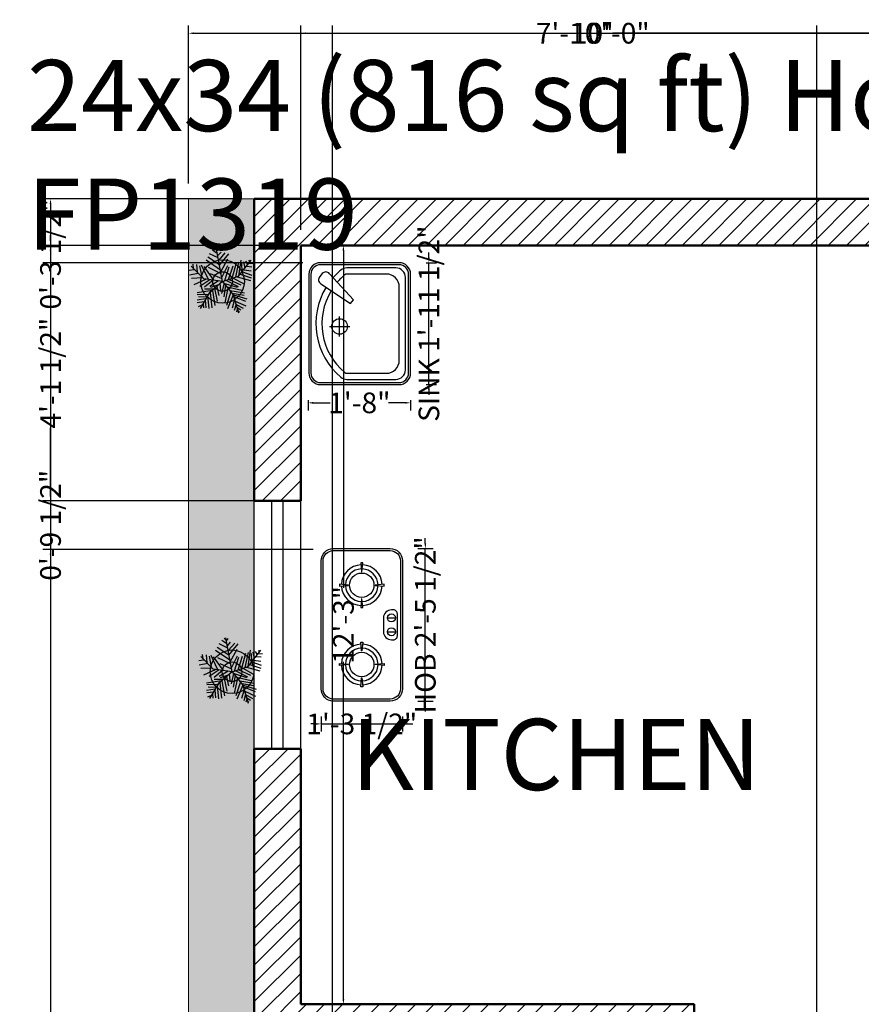
# Model space of a CAD drawing. Units: inches. Extents: x 1265938 to 1266301, y 2357745 to 2358240.
# Tile 3 of 4: x 1265938 to 1266101, y 2358050 to 2358240. Entities that reach past the tile are written whole.
import ezdxf

# ---------------------------------------------------------------- set-up
doc = ezdxf.new("R2010")
doc.units = ezdxf.units.IN
doc.header["$MEASUREMENT"] = 0
for name, color, linetype, lineweight in [('A-ANNO-TEXT', 7, 'Continuous', 25), ('A-AREA-IDEN', 7, 'Continuous', 18), ('A-EQPM', 9, 'Continuous', 25), ('A-FLOR-FIXT', 9, 'Continuous', 25), ('A-WALL-PATT', 8, 'Continuous', 13), ('L-PLNT', 3, 'Continuous', 18), ('L-PLNT-BEDS', 3, 'Continuous', 18), ('L-PLNT-PATT', 3, 'Continuous', 13), ('WALL', 7, 'Continuous', 50), ('WINDOW', 2, 'Continuous', 25), ('YQ_DIM', 3, 'Continuous', 18)]:
    doc.layers.add(name, color=color, linetype=linetype, lineweight=lineweight)
doc.layers.add('Layer2', color=102, linetype='Continuous')
doc.layers.add('RAMP SLOPE', color=8, linetype='Continuous')
doc.styles.get("Standard").update_dxf_attribs({"font": 'arial.ttf'})
doc.styles.add('YQ_DIM', font='SUPEROS.SHX', dxfattribs={"width": 0.8, "bigfont": 'HZDX.SHX'})
doc.dimstyles.new('yqi0', dxfattribs={"dimscale": 0, "dimtxt": 4, "dimasz": 1, "dimexe": 1.5, "dimexo": 3, "dimgap": 0.5, "dimtad": 0, "dimdsep": 46, "dimlunit": 4, "dimtxsty": 'Standard', "dimcen": 0, "dimclrd": 256, "dimclre": 256, "dimclrt": 7, "dimadec": 1, "dimazin": 2, "dimtfac": 1, "dimtix": 1, "dimtmove": 2, "dimatfit": 2, "dimfxl": 1, "dimtolj": 1, "dimtzin": 0, "dimarcsym": 0})

# ---------------------------------------------------------------- blocks, each defined once
blk = doc.blocks.new('*D15')
at = {"layer": 'Defpoints', "color": 0, "transparency": 16777216}
for p in [(1265995.14, 2358196.68), (1265995.14, 2358049.68), (1266001.14, 2358049.68)]:
    blk.add_point(p, dxfattribs=at)
at = {"layer": 'YQ_DIM', "color": 0, "lineweight": -2, "transparency": 16777216}
for p, q in [((1265998.14, 2358196.68), (1266002.64, 2358196.68)), ((1266001.14, 2358195.68), (1266001.14, 2358130.36)), ((1266001.14, 2358050.68), (1266001.14, 2358116)), ((1265998.14, 2358049.68), (1266002.64, 2358049.68))]:
    blk.add_line(p, q, dxfattribs=at)
at = {"layer": 'YQ_DIM', "color": 0, "transparency": 16777216}
for points in [[(1266000.97, 2358195.68), (1266001.31, 2358195.68), (1266001.14, 2358196.68)], [(1266000.97, 2358050.68), (1266001.31, 2358050.68), (1266001.14, 2358049.68)]]:
    blk.add_solid(points, dxfattribs=at)
at = {"layer": 'YQ_DIM', "color": 0, "transparency": 16777216, "insert": (1266001.14, 2358123.18), "char_height": 4, "attachment_point": 5, "rotation": 90}
blk.add_mtext('\\A1;12\'-3"', dxfattribs=at)
blk = doc.blocks.new('WD_WIN4')
for p, q in [((-0.5, 0.5), (0.5, 0.5)), ((-0.5, 0.12), (0.5, 0.12)), ((-0.5, -0.12), (0.5, -0.12)), ((-0.5, -0.5), (0.5, -0.5))]:
    blk.add_line(p, q)
blk = doc.blocks.new('Trees - Metric')
at = {"layer": 'Layer2'}
for p, q in [((-221.9198, 1197.3052), (-433.5526, 1338.8594)), ((-258.7244, 1362.456), (-332.3336, 1421.4348)), ((0, 0), (-266.7, 1447.8)), ((-231.1146, 1315.2628), (-166.7002, 1421.4348)), ((-93.091, 489.5342), (-700.3796, 902.3858)), ((-129.8956, 713.6638), (-626.7704, 1032.1544)), ((-185.1152, 1008.5578), (-553.1612, 1185.4942)), ((-194.31, 1102.9442), (-65.4812, 1256.284)), ((-148.3106, 914.1968), (118.5418, 1220.9018)), ((-129.8956, 701.8528), (265.7602, 1185.4942)), ((-74.7014, 418.7444), (219.7608, 961.39)), ((685.8, 228.6), (1219.2, 914.4)), ((689.0258, 230.0224), (790.2448, 914.1968)), ((983.4626, 867.0036), (1066.2666, 725.4494)), ((1121.4862, 925.9824), (1149.0706, 831.6214)), ((-1206.4492, 501.3198), (-1418.082, 465.9376)), ((-800.1, 114.3), (-1333.5, 647.7)), ((-1234.059, 536.7274), (-1252.4486, 737.2604)), ((-1105.2302, 725.4494), (-1077.6458, 395.1732)), ((-976.4268, 666.4706), (-884.4026, 194.6402)), ((-902.8176, 713.6638), (-617.5756, 100.2538)), ((-369.1382, 53.086), (-783.1836, 642.874)), ((-617.5756, 607.4918), (-74.7014, 347.98)), ((-28.6766, 171.0436), (228.9556, 678.2816)), ((100.1268, 41.275), (284.1498, 619.2774)), ((256.5654, 88.4682), (449.7832, 666.4706)), ((412.9786, 147.447), (587.8068, 796.2392)), ((560.197, 182.8292), (698.2206, 819.8358)), ((808.6344, 784.4282), (827.0494, 418.7444)), ((891.4384, 831.6214), (946.658, 572.1096)), ((919.0482, 501.3198), (1222.6798, 454.152)), ((1029.462, 654.685), (1241.0948, 631.0884)), ((1112.2914, 760.8316), (1296.3144, 784.4282)), ((-1031.621, 347.98), (-1399.667, 277.1902)), ((-847.598, 159.2326), (-1326.0578, 135.636)), ((-718.7946, 88.4682), (-1215.644, -147.447)), ((-543.9664, 76.6572), (-967.2066, -206.4512)), ((0, 0), (-800.1, 114.3)), ((-405.9428, 53.086), (-764.794, -241.8334)), ((0, 0), (-571.5, -495.3)), ((-166.7002, 29.4894), (-543.9664, -206.4512)), ((-525.5514, 347.98), (-28.6766, 123.8504)), ((0, 0), (685.8, 228.6)), ((0, 0), (457.2, -571.5)), ((164.5412, 41.275), (661.416, -218.2368)), ((284.1498, 88.4682), (781.0246, -147.447)), ((458.978, 147.447), (891.4384, -88.4682)), ((615.4166, 194.6402), (1185.8752, 41.275)), ((753.4148, 312.5978), (1222.6798, 159.2326)), ((845.439, 418.7444), (1241.0948, 277.1902)), ((-442.7474, -383.3876), (-1086.8406, -477.7486)), ((-387.5278, -324.4088), (-764.794, -324.4088)), ((-166.7002, -147.447), (-507.1618, -253.619)), ((-433.5526, -383.3876), (-323.1134, -1020.3688)), ((-341.5284, -289.0012), (-221.9198, -831.6214)), ((-240.3094, -218.2368), (-157.5054, -595.7062)), ((-120.7008, -88.4682), (-93.091, -371.5766)), ((63.3222, -76.6826), (-37.8714, -513.1308)), ((44.9326, -64.897), (615.4166, -241.8334)), ((127.7366, -159.258), (54.1274, -654.685)), ((228.9556, -289.0012), (90.932, -914.1968)), ((192.151, -230.0224), (817.8292, -371.5766)), ((311.7596, -383.3876), (937.4378, -477.7486)), ((-718.7946, -737.2604), (-1086.8406, -796.2392)), ((-617.5756, -548.5384), (-1077.6458, -560.324)), ((-681.9646, -666.496), (-1022.4262, -654.685)), ((-571.5, -495.3), (-952.5, -1143)), ((-737.1842, -784.4536), (-709.5744, -1114.7298)), ((-635.9652, -607.5172), (-580.771, -1150.1374)), ((-525.5514, -465.963), (-451.9422, -1126.5408)), ((357.759, -430.5554), (164.5412, -1020.3688)), ((458.978, -572.1096), (210.5406, -1161.923)), ((514.1976, -772.6426), (403.7838, -1138.3264)), ((412.9786, -501.3452), (919.0482, -583.9206)), ((457.2, -571.5), (685.8, -1333.5)), ((468.1982, -572.1096), (1029.462, -737.2604)), ((486.5878, -642.8994), (983.4626, -843.4324)), ((541.8074, -831.6214), (992.6574, -1032.1544)), ((-783.1836, -867.029), (-1077.6458, -902.4112)), ((-875.2078, -1008.5832), (-1040.8412, -1079.3476)), ((-829.2084, -937.7934), (-810.7934, -1126.5408)), ((578.612, -961.39), (495.7826, -1232.7128)), ((578.612, -973.1756), (873.0488, -1138.3264)), ((624.6114, -1161.923), (587.8068, -1291.6916)), ((624.6114, -1102.9442), (781.0246, -1209.1162)), ((679.8056, -1268.095), (716.6102, -1291.6916))]:
    blk.add_line(p, q, dxfattribs=at)
blk = doc.blocks.new('A$Cbdbf8f2b')
at = {"layer": 'RAMP SLOPE'}
for radius in [7.17, 3.22]:
    blk.add_circle((13.77, 14.11), radius, dxfattribs=at)
at = {"xscale": 0.0077264756515533, "yscale": 0.0077264756515533, "zscale": 0.0077264756515533}
blk.add_blockref('Trees - Metric', (13.77, 14.11), dxfattribs=at)
blk = doc.blocks.new('yq_ksink_01')
for points in [[(540, -243.1), (540, 243.1, 0.414214), (483.4, 299.7), (96.6, 299.7, 0.414214), (40, 243.1), (40, -243.1, 0.414214), (96.6, -299.7), (483.4, -299.7, 0.414214)], [(530, -243.1), (530, 243.1, 0.414214), (483.4, 289.7), (96.6, 289.7, 0.414214), (50, 243.1), (50, -243.1, 0.414214), (96.6, -289.7), (483.4, -289.7, 0.414214)], [(141.7, 245.7, 0.463705), (105.6, 245.9), (93.2, 231.4, 0.463199), (98.9, 195.8), (244.3, 98.7), (259.7, 116.6)]]:
    blk.add_lwpolyline(points, format="xyb", close=True)
for points in [[(124.4, 178.8, 0.371537), (197.3, -263.3, 0.175756), (227.1, -274.1), (467.9, -274.1, 0.414214), (514.5, -227.6), (514.5, 227.6, 0.414214), (467.9, 274.1), (227.1, 274.1, 0.175756), (197.3, 263.3, 0.038636), (159.4, 226.3, 0.038636)], [(149.4, 162.1, 0.370424), (216.5, -240.3, 0.175756), (227.1, -244.1), (421.1, -244.1, 0.414214), (484.5, -180.8), (484.5, 180.8, 0.414214), (421.1, 244.1), (227.1, 244.1, 0.175756), (216.5, 240.3, 0.038502), (179.8, 204.1, 0.038502)]]:
    blk.add_lwpolyline(points, format="xyb")
for points in [[(191.1, -63.6), (191.1, 35.7)], [(141.5, -13.9), (240.8, -13.9)]]:
    blk.add_lwpolyline(points)
blk.add_circle((191.1, -13.9), 38.3)
blk = doc.blocks.new('yq_cooker_01')
for p, q in [((426.3, 34.3), (465.5, 34.3)), ((426.3, -34.3), (465.5, -34.3))]:
    blk.add_line(p, q)
for points in [[(440, -375), (160, -375, -0.414214), (100, -315), (100, 315, -0.414214), (160, 375), (440, 375, -0.414214), (500, 315), (500, -315, -0.414214)], [(440, -365), (160, -365, -0.414214), (110, -315), (110, 315, -0.414214), (160, 365), (440, 365, -0.414214), (490, 315), (490, -315, -0.414214)]]:
    blk.add_lwpolyline(points, format="xyb", close=True)
for points in [[(300.8, 261.3), (305.4, 305), (294.6, 305), (299.2, 261.3)], [(233.7, 195.8), (190, 200.4), (190, 189.6), (233.7, 194.2)], [(366.3, 194.2), (410, 189.6), (410, 200.4), (366.3, 195.8)], [(299.2, 128.7), (294.6, 85), (305.4, 85), (300.8, 128.7)], [(299.2, -128.7), (294.6, -85), (305.4, -85), (300.8, -128.7)], [(233.7, -195.8), (190, -200.4), (190, -189.6), (233.7, -194.2)], [(366.3, -194.2), (410, -189.6), (410, -200.4), (366.3, -195.8)], [(300.8, -261.3), (305.4, -305), (294.6, -305), (299.2, -261.3)]]:
    blk.add_lwpolyline(points, close=True)
blk.add_lwpolyline([(406.7, -34.3, 0.414214), (445.9, -73.5), (455.5, -73.5, 0.414214), (475.1, -53.9), (475.1, 53.9, 0.414214), (455.5, 73.5), (445.9, 73.5, 0.414214), (406.7, 34.3), (406.7, -34.3)], format="xyb")
for centre, radius in [((300, 195), 60), ((445.9, 34.3), 19.6), ((445.9, -34.3), 19.6), ((300, -195), 60)]:
    blk.add_circle(centre, radius)
for centre, radius, start, end in [((300, 195), 100, 92.4978, 177.5022), ((300, 195), 100, 2.4978, 87.5022), ((300, 195), 80, 91.5913, 178.4087), ((300, 195), 80, 1.5913, 88.4087), ((300, 195), 100, 182.4978, 267.5022), ((300, 195), 80, 181.5913, 268.4087), ((300, 195), 80, 271.5913, 358.4087), ((300, 195), 100, 272.4978, 357.5022), ((300, -195), 100, 92.4978, 177.5022), ((300, -195), 100, 2.4978, 87.5022), ((300, -195), 80, 91.5913, 178.4087), ((300, -195), 80, 1.5913, 88.4087), ((300, -195), 100, 182.4978, 267.5022), ((300, -195), 80, 181.5913, 268.4087), ((300, -195), 80, 271.5913, 358.4087), ((300, -195), 100, 272.4978, 357.5022)]:
    blk.add_arc(centre, radius, start, end)
blk = doc.blocks.new('*D30')
at = {"layer": 'Defpoints', "color": 0, "transparency": 16777216}
for p in [(1266012.58, 2358137.94), (1266017, 2358137.94), (1266012.58, 2358108.42)]:
    blk.add_point(p, dxfattribs=at)
at = {"layer": 'YQ_DIM', "lineweight": -2, "transparency": 16777216}
for p, q in [((1266017, 2358138.94), (1266017, 2358139.94)), ((1266015.58, 2358137.94), (1266018.5, 2358137.94)), ((1266017, 2358108.42), (1266017, 2358137.94)), ((1266015.58, 2358108.42), (1266018.5, 2358108.42)), ((1266017, 2358107.42), (1266017, 2358106.42))]:
    blk.add_line(p, q, dxfattribs=at)
at = {"layer": 'YQ_DIM', "transparency": 16777216}
for points in [[(1266016.84, 2358138.94), (1266017.17, 2358138.94), (1266017, 2358137.94)], [(1266016.84, 2358107.42), (1266017.17, 2358107.42), (1266017, 2358108.42)]]:
    blk.add_solid(points, dxfattribs=at)
at = {"layer": 'YQ_DIM', "color": 7, "transparency": 16777216, "insert": (1266017, 2358123.18), "char_height": 4, "attachment_point": 5, "rotation": 90}
blk.add_mtext('\\A1;HOB 2\'-5 1/2"', dxfattribs=at)
blk = doc.blocks.new('*D31')
at = {"layer": 'Defpoints', "color": 0, "transparency": 16777216}
for p in [(1265996.83, 2358108.42), (1266012.58, 2358108.42), (1266012.58, 2358103.99)]:
    blk.add_point(p, dxfattribs=at)
at = {"layer": 'YQ_DIM', "lineweight": -2, "transparency": 16777216}
for p, q in [((1265996.83, 2358105.42), (1265996.83, 2358102.49)), ((1266012.58, 2358105.42), (1266012.58, 2358102.49)), ((1265995.83, 2358103.99), (1265994.83, 2358103.99)), ((1265996.83, 2358103.99), (1266012.58, 2358103.99)), ((1266013.58, 2358103.99), (1266014.58, 2358103.99))]:
    blk.add_line(p, q, dxfattribs=at)
at = {"layer": 'YQ_DIM', "transparency": 16777216}
for points in [[(1265995.83, 2358104.15), (1265995.83, 2358103.82), (1265996.83, 2358103.99)], [(1266013.58, 2358104.15), (1266013.58, 2358103.82), (1266012.58, 2358103.99)]]:
    blk.add_solid(points, dxfattribs=at)
at = {"layer": 'YQ_DIM', "color": 7, "transparency": 16777216, "insert": (1266004.7, 2358103.99), "char_height": 4, "attachment_point": 5}
blk.add_mtext('\\A1;1\'-3 1/2"', dxfattribs=at)
blk = doc.blocks.new('*D32')
at = {"layer": 'Defpoints', "color": 0, "transparency": 16777216}
for p in [(1266014.15, 2358193.32), (1266017.69, 2358193.32), (1266014.15, 2358169.72)]:
    blk.add_point(p, dxfattribs=at)
at = {"layer": 'YQ_DIM', "lineweight": -2, "transparency": 16777216}
for p, q in [((1266017.69, 2358194.32), (1266017.69, 2358195.32)), ((1266017.15, 2358193.32), (1266019.19, 2358193.32)), ((1266017.69, 2358169.72), (1266017.69, 2358193.32)), ((1266017.15, 2358169.72), (1266019.19, 2358169.72)), ((1266017.69, 2358168.72), (1266017.69, 2358167.72))]:
    blk.add_line(p, q, dxfattribs=at)
at = {"layer": 'YQ_DIM', "transparency": 16777216}
for points in [[(1266017.52, 2358194.32), (1266017.86, 2358194.32), (1266017.69, 2358193.32)], [(1266017.52, 2358168.72), (1266017.86, 2358168.72), (1266017.69, 2358169.72)]]:
    blk.add_solid(points, dxfattribs=at)
at = {"layer": 'YQ_DIM', "color": 7, "transparency": 16777216, "insert": (1266017.69, 2358181.52), "char_height": 4, "attachment_point": 5, "rotation": 90}
blk.add_mtext('\\A1;SINK 1\'-11 1/2"', dxfattribs=at)
blk = doc.blocks.new('*D33')
at = {"layer": 'Defpoints', "color": 0, "transparency": 16777216}
for p in [(1265994.3, 2358169.72), (1266014.15, 2358169.72), (1266014.15, 2358166.18)]:
    blk.add_point(p, dxfattribs=at)
at = {"layer": 'YQ_DIM', "lineweight": -2, "transparency": 16777216}
for p, q in [((1265994.3, 2358166.72), (1265994.3, 2358164.68)), ((1265995.3, 2358166.18), (1265998.6, 2358166.18)), ((1266013.15, 2358166.18), (1266009.85, 2358166.18)), ((1266014.15, 2358166.72), (1266014.15, 2358164.68))]:
    blk.add_line(p, q, dxfattribs=at)
at = {"layer": 'YQ_DIM', "transparency": 16777216}
for points in [[(1265995.3, 2358166.35), (1265995.3, 2358166.02), (1265994.3, 2358166.18)], [(1266013.15, 2358166.35), (1266013.15, 2358166.02), (1266014.15, 2358166.18)]]:
    blk.add_solid(points, dxfattribs=at)
at = {"layer": 'YQ_DIM', "color": 7, "transparency": 16777216, "insert": (1266004.23, 2358166.18), "char_height": 4, "attachment_point": 5}
blk.add_mtext('\\A1;1\'-8"', dxfattribs=at)
blk = doc.blocks.new('*D34')
at = {"layer": 'Defpoints', "color": 0, "transparency": 16777216}
for p in [(1266259.14, 2358237.77), (1265971.14, 2358205.68), (1266259.14, 2358205.68)]:
    blk.add_point(p, dxfattribs=at)
at = {"layer": 'YQ_DIM', "lineweight": -2, "transparency": 16777216}
for p, q in [((1265971.14, 2358208.68), (1265971.14, 2358239.27)), ((1266259.14, 2358208.68), (1266259.14, 2358239.27)), ((1265972.14, 2358237.77), (1266107.74, 2358237.77)), ((1266258.14, 2358237.77), (1266122.54, 2358237.77))]:
    blk.add_line(p, q, dxfattribs=at)
at = {"layer": 'YQ_DIM', "transparency": 16777216}
for points in [[(1265972.14, 2358237.93), (1265972.14, 2358237.6), (1265971.14, 2358237.77)], [(1266258.14, 2358237.93), (1266258.14, 2358237.6), (1266259.14, 2358237.77)]]:
    blk.add_solid(points, dxfattribs=at)
at = {"layer": 'YQ_DIM', "color": 7, "transparency": 16777216, "insert": (1266115.14, 2358237.77), "char_height": 4, "attachment_point": 5}
blk.add_mtext('\\A1;24\'-0"', dxfattribs=at)
blk = doc.blocks.new('*D37')
at = {"layer": 'Defpoints', "color": 0, "transparency": 16777216}
for p in [(1265944.45, 2358205.68), (1265983.89, 2358205.68), (1265983.89, 2357809.68)]:
    blk.add_point(p, dxfattribs=at)
at = {"layer": 'YQ_DIM', "lineweight": -2, "transparency": 16777216}
for p, q in [((1265980.89, 2358205.68), (1265942.95, 2358205.68)), ((1265944.45, 2358204.68), (1265944.45, 2358015.05)), ((1265944.45, 2357810.68), (1265944.45, 2358000.31)), ((1265980.89, 2357809.68), (1265942.95, 2357809.68))]:
    blk.add_line(p, q, dxfattribs=at)
at = {"layer": 'YQ_DIM', "transparency": 16777216}
for points in [[(1265944.29, 2358204.68), (1265944.62, 2358204.68), (1265944.45, 2358205.68)], [(1265944.29, 2357810.68), (1265944.62, 2357810.68), (1265944.45, 2357809.68)]]:
    blk.add_solid(points, dxfattribs=at)
at = {"layer": 'YQ_DIM', "color": 7, "transparency": 16777216, "insert": (1265944.45, 2358007.68), "char_height": 4, "attachment_point": 5, "rotation": 90}
blk.add_mtext('\\A1;33\'-0"', dxfattribs=at)
blk = doc.blocks.new('*D38')
at = {"layer": 'Defpoints', "color": 0, "transparency": 16777216}
for p in [(1266112.89, 2358237.77), (1265992.89, 2358196.68), (1266112.89, 2358196.68)]:
    blk.add_point(p, dxfattribs=at)
at = {"layer": 'YQ_DIM', "lineweight": -2, "transparency": 16777216}
for p, q in [((1265992.89, 2358199.68), (1265992.89, 2358239.27)), ((1266112.89, 2358199.68), (1266112.89, 2358239.27)), ((1265993.89, 2358237.77), (1266045.71, 2358237.77)), ((1266111.89, 2358237.77), (1266060.07, 2358237.77))]:
    blk.add_line(p, q, dxfattribs=at)
at = {"layer": 'YQ_DIM', "transparency": 16777216}
for points in [[(1265993.89, 2358237.93), (1265993.89, 2358237.6), (1265992.89, 2358237.77)], [(1266111.89, 2358237.93), (1266111.89, 2358237.6), (1266112.89, 2358237.77)]]:
    blk.add_solid(points, dxfattribs=at)
at = {"layer": 'YQ_DIM', "color": 7, "transparency": 16777216, "insert": (1266052.89, 2358237.77), "char_height": 4, "attachment_point": 5}
blk.add_mtext('\\A1;10\'-0"', dxfattribs=at)
blk = doc.blocks.new('*D45')
at = {"layer": 'Defpoints', "color": 0, "transparency": 16777216}
for p in [(1265992.89, 2358196.68), (1265944.45, 2358147.18), (1265992.89, 2358147.18)]:
    blk.add_point(p, dxfattribs=at)
at = {"layer": 'YQ_DIM', "lineweight": -2, "transparency": 16777216}
for p, q in [((1265989.89, 2358196.68), (1265942.95, 2358196.68)), ((1265944.45, 2358195.68), (1265944.45, 2358182.49)), ((1265944.45, 2358148.18), (1265944.45, 2358161.37)), ((1265989.89, 2358147.18), (1265942.95, 2358147.18))]:
    blk.add_line(p, q, dxfattribs=at)
at = {"layer": 'YQ_DIM', "transparency": 16777216}
for points in [[(1265944.29, 2358195.68), (1265944.62, 2358195.68), (1265944.45, 2358196.68)], [(1265944.29, 2358148.18), (1265944.62, 2358148.18), (1265944.45, 2358147.18)]]:
    blk.add_solid(points, dxfattribs=at)
at = {"layer": 'YQ_DIM', "color": 7, "transparency": 16777216, "insert": (1265944.45, 2358171.93), "char_height": 4, "attachment_point": 5, "rotation": 90}
blk.add_mtext('\\A1;4\'-1 1/2"', dxfattribs=at)
blk = doc.blocks.new('*D55')
at = {"layer": 'Defpoints', "color": 0, "transparency": 16777216}
for p in [(1266092.81, 2358237.77), (1265999.06, 2357848.06), (1266092.81, 2357848.06)]:
    blk.add_point(p, dxfattribs=at)
at = {"layer": 'YQ_DIM', "lineweight": -2, "transparency": 16777216}
for p, q in [((1265999.06, 2357851.06), (1265999.06, 2358239.27)), ((1266092.81, 2357851.06), (1266092.81, 2358239.27)), ((1266000.06, 2358237.77), (1266038.58, 2358237.77)), ((1266091.81, 2358237.77), (1266053.28, 2358237.77))]:
    blk.add_line(p, q, dxfattribs=at)
at = {"layer": 'YQ_DIM', "transparency": 16777216}
for points in [[(1266000.06, 2358237.93), (1266000.06, 2358237.6), (1265999.06, 2358237.77)], [(1266091.81, 2358237.93), (1266091.81, 2358237.6), (1266092.81, 2358237.77)]]:
    blk.add_solid(points, dxfattribs=at)
at = {"layer": 'YQ_DIM', "color": 7, "transparency": 16777216, "insert": (1266045.93, 2358237.77), "char_height": 4, "attachment_point": 5}
blk.add_mtext('\\A1;7\'-10"', dxfattribs=at)
blk = doc.blocks.new('*D60')
at = {"layer": 'Defpoints', "color": 0, "transparency": 16777216}
for p in [(1265992.89, 2358196.68), (1265944.45, 2358193.27), (1265996.26, 2358193.27)]:
    blk.add_point(p, dxfattribs=at)
at = {"layer": 'YQ_DIM', "lineweight": -2, "transparency": 16777216}
for p, q in [((1265944.45, 2358197.68), (1265944.45, 2358198.68)), ((1265989.89, 2358196.68), (1265942.95, 2358196.68)), ((1265944.45, 2358196.68), (1265944.45, 2358193.27)), ((1265993.26, 2358193.27), (1265942.95, 2358193.27)), ((1265944.45, 2358192.27), (1265944.45, 2358191.27))]:
    blk.add_line(p, q, dxfattribs=at)
at = {"layer": 'YQ_DIM', "transparency": 16777216}
for points in [[(1265944.29, 2358197.68), (1265944.62, 2358197.68), (1265944.45, 2358196.68)], [(1265944.29, 2358192.27), (1265944.62, 2358192.27), (1265944.45, 2358193.27)]]:
    blk.add_solid(points, dxfattribs=at)
at = {"layer": 'YQ_DIM', "color": 7, "transparency": 16777216, "insert": (1265944.45, 2358194.98), "char_height": 4, "attachment_point": 5, "rotation": 90}
blk.add_mtext('\\A1;0\'-3 1/2"', dxfattribs=at)
blk = doc.blocks.new('*D61')
at = {"layer": 'Defpoints', "color": 0, "transparency": 16777216}
for p in [(1265992.89, 2358147.18), (1265944.45, 2358137.76), (1265998.27, 2358137.76)]:
    blk.add_point(p, dxfattribs=at)
at = {"layer": 'YQ_DIM', "lineweight": -2, "transparency": 16777216}
for p, q in [((1265944.45, 2358148.18), (1265944.45, 2358149.18)), ((1265989.89, 2358147.18), (1265942.95, 2358147.18)), ((1265944.45, 2358147.18), (1265944.45, 2358137.76)), ((1265995.27, 2358137.76), (1265942.95, 2358137.76)), ((1265944.45, 2358136.76), (1265944.45, 2358135.76))]:
    blk.add_line(p, q, dxfattribs=at)
at = {"layer": 'YQ_DIM', "transparency": 16777216}
for points in [[(1265944.29, 2358148.18), (1265944.62, 2358148.18), (1265944.45, 2358147.18)], [(1265944.29, 2358136.76), (1265944.62, 2358136.76), (1265944.45, 2358137.76)]]:
    blk.add_solid(points, dxfattribs=at)
at = {"layer": 'YQ_DIM', "color": 7, "transparency": 16777216, "insert": (1265944.45, 2358142.47), "char_height": 4, "attachment_point": 5, "rotation": 90}
blk.add_mtext('\\A1;0\'-9 1/2"', dxfattribs=at)

msp = doc.modelspace()

# ---------------------------------------------------------------- hatches: boundary and pattern name
at = {"layer": 'A-WALL-PATT'}
h = msp.add_hatch(dxfattribs=at)
h.set_pattern_fill('ANSI31', color=256, scale=20)
h.paths.add_polyline_path([(1266246.39, 2358205.681), (1265983.89, 2358205.681), (1265983.89, 2358147.181), (1265992.89, 2358147.181), (1265992.89, 2358196.681), (1266112.89, 2358196.681), (1266119.229, 2358196.681), (1266237.39, 2358196.681), (1266237.39, 2358147.181), (1266246.39, 2358147.181)])
h = msp.add_hatch(dxfattribs=at)
h.set_pattern_fill('ANSI31', color=256, scale=20)
h.paths.add_polyline_path([(1266069.016, 2358049.681), (1265992.89, 2358049.681), (1265992.89, 2358099.181), (1265983.89, 2358099.181), (1265983.89, 2358012.181), (1265992.89, 2358012.181), (1265992.89, 2358045.181), (1266069.016, 2358045.181)])
h.paths.add_polyline_path([(1266246.39, 2358049.681), (1266246.39, 2358099.181), (1266237.39, 2358099.181), (1266237.39, 2358049.681), (1266161.264, 2358049.681), (1266161.264, 2358045.181), (1266178.89, 2358045.181), (1266178.89, 2357987.055), (1266183.39, 2357987.055), (1266183.39, 2358045.181), (1266237.39, 2358045.181), (1266237.39, 2358029.655), (1266246.39, 2358029.655)])
h.paths.add_polyline_path([(1265992.89, 2357938.681), (1266058.89, 2357938.681), (1266058.89, 2357943.181), (1265992.89, 2357943.181), (1265992.89, 2357976.181), (1265983.89, 2357976.181), (1265983.89, 2357967.701), (1265984.307, 2357966.989), (1265983.89, 2357967.035), (1265983.89, 2357902.681), (1265992.89, 2357902.681)])
h.paths.add_polyline_path([(1266069.016, 2357943.181), (1266058.89, 2357943.181), (1266058.89, 2357938.681), (1266069.016, 2357938.681)])
h.paths.add_polyline_path([(1266125.264, 2357943.181), (1266105.016, 2357943.181), (1266105.016, 2357938.681), (1266112.89, 2357938.681), (1266112.89, 2357818.681), (1266105.024, 2357818.681), (1266105.024, 2357809.681), (1266112.898, 2357809.681), (1266153.39, 2357809.681), (1266153.39, 2357818.681), (1266117.39, 2357818.681), (1266117.39, 2357938.681), (1266125.264, 2357938.681)])
h.paths.add_polyline_path([(1266069.024, 2357818.681), (1265999.055, 2357818.681), (1265992.89, 2357818.681), (1265992.89, 2357854.681), (1265983.89, 2357854.681), (1265983.89, 2357809.681), (1266069.024, 2357809.681)])
h.paths.add_polyline_path([(1266246.39, 2358005.655), (1266237.39, 2358005.655), (1266237.39, 2357943.181), (1266161.264, 2357943.181), (1266161.264, 2357938.681), (1266237.39, 2357938.681), (1266237.39, 2357818.681), (1266201.39, 2357818.681), (1266201.39, 2357809.681), (1266246.39, 2357809.681)])
at = {"layer": 'L-PLNT-PATT'}
h = msp.add_hatch(dxfattribs=at)
h.set_pattern_fill('GRASS', color=256, scale=4)
h.paths.add_polyline_path([(1265983.89, 2358205.681), (1265971.14, 2358205.681), (1265971.14, 2357797.681), (1265983.89, 2357797.681)])

# ---------------------------------------------------------------- linework, layer by layer
at = {"layer": 'L-PLNT-BEDS'}
msp.add_lwpolyline([(1265971.14, 2357797.681), (1265971.14, 2358205.681), (1265983.89, 2358205.681), (1265983.89, 2357797.681)], close=True, dxfattribs=at)
at = {"layer": 'WALL'}
for p, q in [((1265983.89, 2358147.181), (1265983.89, 2358205.681)), ((1265992.89, 2358196.681), (1266112.89, 2358196.681)), ((1265992.89, 2358147.181), (1265992.89, 2358196.681)), ((1265992.89, 2358147.181), (1265983.89, 2358147.181)), ((1265992.89, 2358099.181), (1265983.89, 2358099.181)), ((1265983.89, 2358012.181), (1265983.89, 2358099.181)), ((1265992.89, 2358049.681), (1265992.89, 2358099.181)), ((1265992.89, 2358049.681), (1266069.016, 2358049.681)), ((1266069.016, 2358049.681), (1266069.016, 2358045.181))]:
    msp.add_line(p, q, dxfattribs=at)
msp.add_lwpolyline([(1265983.89, 2358205.681), (1266246.39, 2358205.681)], dxfattribs=at)

# ---------------------------------------------------------------- block references
at = {"layer": 'A-EQPM', "xscale": 0.0393700787401575, "yscale": 0.0393700787401575, "zscale": 0.0393700787401575}
msp.add_blockref('yq_cooker_01', (1265992.89, 2358123.181), dxfattribs=at)
at = {"layer": 'A-FLOR-FIXT', "xscale": 0.0393700787401575, "yscale": 0.0393700787401575, "zscale": 0.0393700787401575}
msp.add_blockref('yq_ksink_01', (1265992.89, 2358181.52), dxfattribs=at)
at = {"layer": 'L-PLNT', "xscale": 0.5886644209444821, "yscale": 0.5886644209444821, "zscale": 0.5886644209444821}
for p in [(1265969.644, 2358181.373), (1265971.482, 2358105.782)]:
    msp.add_blockref('A$Cbdbf8f2b', p, dxfattribs=at)
at = {"layer": 'WINDOW', "xscale": 48, "yscale": 9, "zscale": 48, "rotation": 90}
msp.add_blockref('WD_WIN4', (1265988.39, 2358123.181), dxfattribs=at)

# ---------------------------------------------------------------- texts
at = {"layer": 'A-ANNO-TEXT', "insert": (1265939.922, 2358232.591), "char_height": 13.77953, "width": 415.35736, "attachment_point": 1, "style": 'YQ_DIM'}
msp.add_mtext('24x34 (816 sq ft) House Plan - North face - FP1319', dxfattribs=at)
at = {"layer": 'A-AREA-IDEN', "insert": (1266013.615, 2358104.961), "char_height": 13.77953, "width": 57.36631, "attachment_point": 1, "style": 'YQ_DIM'}
msp.add_mtext('\\pxqc;KITCHEN', dxfattribs=at)

# ---------------------------------------------------------------- dimensions: what is measured, and where the dimension line sits
at = {"layer": 'YQ_DIM'}
for base, p1, p2, picture, middle in [((1266259.14, 2358237.768), (1265971.14, 2358205.681), (1266259.14, 2358205.681), '*D34', (1266115.14, 2358237.768)), ((1266112.89, 2358237.768), (1265992.89, 2358196.681), (1266112.89, 2358196.681), '*D38', (1266052.89, 2358237.768)), ((1266092.80533, 2358237.768232), (1265999.05533, 2357848.055565), (1266092.80533, 2357848.055565), '*D55', (1266045.93033, 2358237.768232)), ((1266014.15, 2358166.183), (1265994.301, 2358169.723), (1266014.15, 2358169.723), '*D33', (1266004.226, 2358166.183)), ((1266012.575, 2358103.988), (1265996.827, 2358108.417), (1266012.575, 2358108.417), '*D31', (1266004.701, 2358103.988))]:
    dim = msp.add_linear_dim(base=base, p1=p1, p2=p2, dimstyle='yqi0', override={"dimscale": 1, "dimdec": 1, "dimzin": 1, "dimfrac": 2}, dxfattribs=at)
    dim.commit()
    dim.dimension.update_dxf_attribs({"geometry": picture, "text_midpoint": middle})
for base, p1, p2, angle, override, picture, middle in [((1265944.452, 2358193.274), (1265992.89, 2358196.681), (1265996.255, 2358193.274), 90, {"dimscale": 1, "dimdec": 1, "dimzin": 1, "dimfrac": 2}, '*D60', (1265944.452, 2358194.977)), ((1265944.452, 2358205.681), (1265983.89, 2357809.681), (1265983.89, 2358205.681), 90, {"dimscale": 1, "dimdec": 1, "dimzin": 1, "dimfrac": 2}, '*D37', (1265944.452, 2358007.681)), ((1265944.452, 2358147.181), (1265992.89, 2358196.681), (1265992.89, 2358147.181), 90, {"dimscale": 1, "dimdec": 1, "dimzin": 1, "dimfrac": 2}, '*D45', (1265944.452, 2358171.931)), ((1266001.14, 2358049.681), (1265995.14, 2358196.681), (1265995.14, 2358049.681), 270, {"dimscale": 1, "dimclrd": 0, "dimclre": 0, "dimclrt": 0}, '*D15', (1266001.14, 2358123.181)), ((1265944.452, 2358137.759), (1265992.89, 2358147.181), (1265998.27, 2358137.759), 90, {"dimscale": 1, "dimdec": 1, "dimzin": 1, "dimfrac": 2}, '*D61', (1265944.452, 2358142.47))]:
    dim = msp.add_linear_dim(base=base, p1=p1, p2=p2, angle=angle, dimstyle='yqi0', override=override, dxfattribs=at)
    dim.commit()
    dim.dimension.update_dxf_attribs({"geometry": picture, "text_midpoint": middle})
for base, p1, p2, text, picture, middle in [((1266017.69, 2358193.317), (1266014.15, 2358169.723), (1266014.15, 2358193.317), 'SINK <>', '*D32', (1266017.69, 2358181.52)), ((1266017.005, 2358137.944), (1266012.575, 2358108.417), (1266012.575, 2358137.944), 'HOB <>', '*D30', (1266017.005, 2358123.181))]:
    dim = msp.add_linear_dim(base=base, p1=p1, p2=p2, angle=90, text=text, dimstyle='yqi0', override={"dimscale": 1, "dimdec": 1, "dimzin": 1, "dimfrac": 2}, dxfattribs=at)
    dim.commit()
    dim.dimension.update_dxf_attribs({"geometry": picture, "text_midpoint": middle})

doc.saveas('drawing.dxf')
